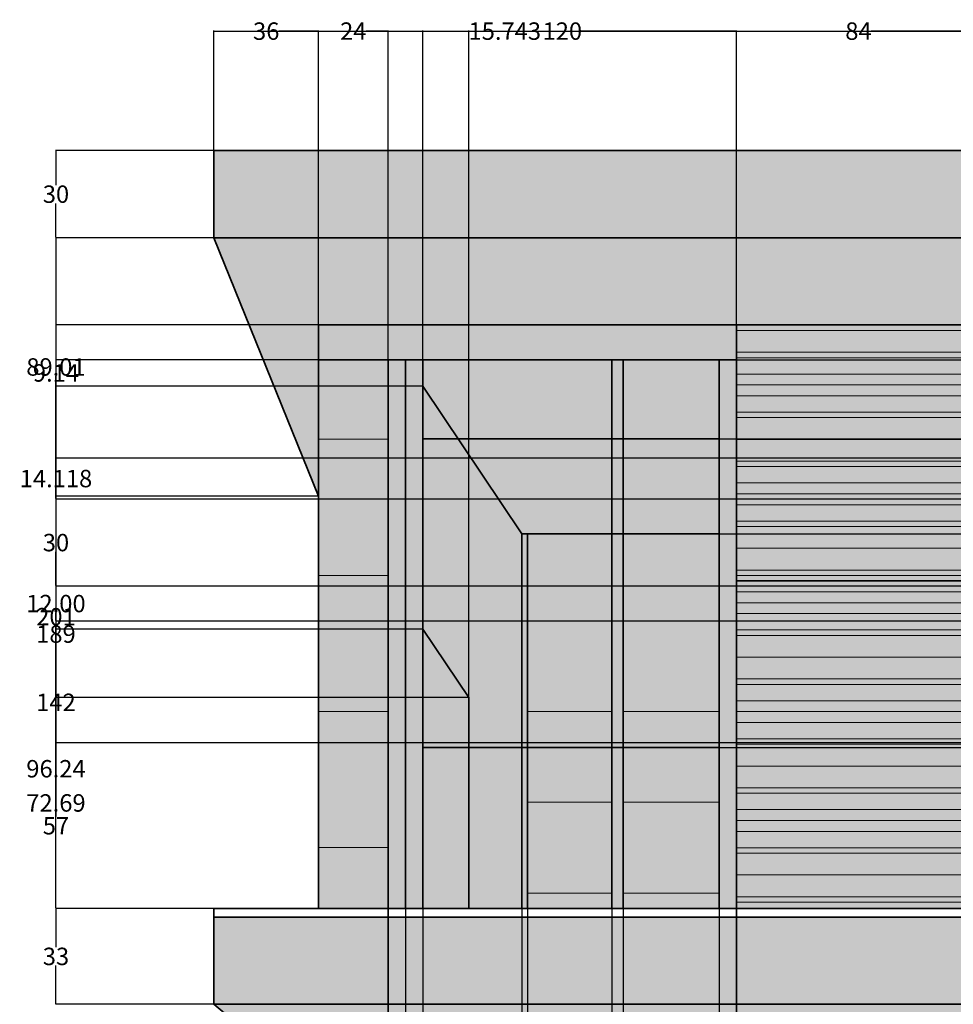
# Model space of a CAD drawing. Units: inches. Extents: x 148 to 1080, y 89 to 707.
# Tile 6 of 12: x 148 to 470, y 368 to 707. Entities that reach past the tile are written whole.
import ezdxf

# ---------------------------------------------------------------- set-up
doc = ezdxf.new("R2010")
doc.units = ezdxf.units.IN
doc.header["$MEASUREMENT"] = 0
for name, color, linetype, lineweight in [('A-ANNO-DIMS', 2, 'Continuous', 18), ('A-ELEV', 7, 'Continuous', 35), ('A-ELEV-PATT', 8, 'Continuous', 13)]:
    doc.layers.add(name, color=color, linetype=linetype, lineweight=lineweight)
doc.styles.get("Standard").update_dxf_attribs({"font": 'arial.ttf'})
doc.dimstyles.get("Standard").update_dxf_attribs({"dimtxt": 6, "dimasz": 0.18, "dimexe": 0.18, "dimexo": 0.0625, "dimgap": 0.09, "dimtad": 0, "dimtih": 1, "dimtoh": 1, "dimdec": 0, "dimzin": 0, "dimdsep": 46, "dimlunit": 3, "dimtxsty": 'Standard', "dimcen": 0.09, "dimadec": 0, "dimazin": 0, "dimtfac": 1, "dimtdec": 0, "dimtofl": 0, "dimtmove": 0, "dimatfit": 3, "dimfxl": 1, "dimtolj": 1, "dimtzin": 0, "dimarcsym": 0})

# ---------------------------------------------------------------- blocks, each defined once
blk = doc.blocks.new('*D1')
at = {"layer": 'A-ANNO-DIMS', "color": 0, "lineweight": -2, "transparency": 16777216}
for p, q in [((215.02, 662.01), (215.02, 703.28)), ((215.2, 703.1), (604.32, 703.1)), ((1006.77, 703.1), (617.65, 703.1)), ((1006.95, 338.01), (1006.95, 703.28))]:
    blk.add_line(p, q, dxfattribs=at)
at = {"layer": 'A-ANNO-DIMS', "color": 0, "transparency": 16777216}
for points in [[(215.2, 703.13), (215.2, 703.07), (215.02, 703.1)], [(1006.77, 703.13), (1006.77, 703.07), (1006.95, 703.1)]]:
    blk.add_solid(points, dxfattribs=at)
at = {"layer": 'Defpoints', "color": 0, "transparency": 16777216}
for p in [(1006.95, 703.1), (215.02, 661.95), (1006.95, 337.95)]:
    blk.add_point(p, dxfattribs=at)
at = {"layer": 'A-ANNO-DIMS', "color": 0, "transparency": 16777216, "insert": (610.98, 703.1), "char_height": 6, "attachment_point": 5}
blk.add_mtext('\\A1;792', dxfattribs=at)
blk = doc.blocks.new('*D8')
at = {"layer": 'A-ANNO-DIMS', "color": 0, "lineweight": -2, "transparency": 16777216}
for p, q in [((215.02, 632.01), (215.02, 703.28)), ((215.2, 703.1), (228.64, 703.1)), ((250.84, 703.1), (237.4, 703.1)), ((251.02, 543), (251.02, 703.28))]:
    blk.add_line(p, q, dxfattribs=at)
at = {"layer": 'A-ANNO-DIMS', "color": 0, "transparency": 16777216}
for points in [[(215.2, 703.13), (215.2, 703.07), (215.02, 703.1)], [(250.84, 703.13), (250.84, 703.07), (251.02, 703.1)]]:
    blk.add_solid(points, dxfattribs=at)
at = {"layer": 'Defpoints', "color": 0, "transparency": 16777216}
for p in [(251.02, 703.1), (215.02, 631.95), (251.02, 542.94)]:
    blk.add_point(p, dxfattribs=at)
at = {"layer": 'A-ANNO-DIMS', "color": 0, "transparency": 16777216, "insert": (233.02, 703.1), "char_height": 6, "attachment_point": 5}
blk.add_mtext('\\A1;36', dxfattribs=at)
blk = doc.blocks.new('*D9')
at = {"layer": 'A-ANNO-DIMS', "color": 0, "lineweight": -2, "transparency": 16777216}
for p, q in [((251.02, 602.01), (251.02, 703.28)), ((251.2, 703.1), (258.59, 703.1)), ((274.84, 703.1), (267.45, 703.1)), ((275.02, 590.01), (275.02, 703.28))]:
    blk.add_line(p, q, dxfattribs=at)
at = {"layer": 'A-ANNO-DIMS', "color": 0, "transparency": 16777216}
for points in [[(251.2, 703.13), (251.2, 703.07), (251.02, 703.1)], [(274.84, 703.13), (274.84, 703.07), (275.02, 703.1)]]:
    blk.add_solid(points, dxfattribs=at)
at = {"layer": 'Defpoints', "color": 0, "transparency": 16777216}
for p in [(275.02, 703.1), (251.02, 601.95), (275.02, 589.95)]:
    blk.add_point(p, dxfattribs=at)
at = {"layer": 'A-ANNO-DIMS', "color": 0, "transparency": 16777216, "insert": (263.02, 703.1), "char_height": 6, "attachment_point": 5}
blk.add_mtext('\\A1;24', dxfattribs=at)
blk = doc.blocks.new('*D10')
at = {"layer": 'A-ANNO-DIMS', "color": 0, "lineweight": -2, "transparency": 16777216}
for p, q in [((275.02, 590.01), (275.02, 703.28)), ((275.2, 703.1), (328.59, 703.1)), ((394.84, 703.1), (341.45, 703.1)), ((395.02, 590.01), (395.02, 703.28))]:
    blk.add_line(p, q, dxfattribs=at)
at = {"layer": 'A-ANNO-DIMS', "color": 0, "transparency": 16777216}
for points in [[(275.2, 703.13), (275.2, 703.07), (275.02, 703.1)], [(394.84, 703.13), (394.84, 703.07), (395.02, 703.1)]]:
    blk.add_solid(points, dxfattribs=at)
at = {"layer": 'Defpoints', "color": 0, "transparency": 16777216}
for p in [(395.02, 703.1), (275.02, 589.95), (395.02, 589.95)]:
    blk.add_point(p, dxfattribs=at)
at = {"layer": 'A-ANNO-DIMS', "color": 0, "transparency": 16777216, "insert": (335.02, 703.1), "char_height": 6, "attachment_point": 5}
blk.add_mtext('\\A1;120', dxfattribs=at)
blk = doc.blocks.new('*D11')
at = {"layer": 'A-ANNO-DIMS', "color": 0, "lineweight": -2, "transparency": 16777216}
for p, q in [((395.02, 602.01), (395.02, 703.28)), ((395.2, 703.1), (432.64, 703.1)), ((478.84, 703.1), (441.4, 703.1)), ((479.02, 602.01), (479.02, 703.28))]:
    blk.add_line(p, q, dxfattribs=at)
at = {"layer": 'A-ANNO-DIMS', "color": 0, "transparency": 16777216}
for points in [[(395.2, 703.13), (395.2, 703.07), (395.02, 703.1)], [(478.84, 703.13), (478.84, 703.07), (479.02, 703.1)]]:
    blk.add_solid(points, dxfattribs=at)
at = {"layer": 'Defpoints', "color": 0, "transparency": 16777216}
for p in [(479.02, 703.1), (395.02, 601.95), (479.02, 601.95)]:
    blk.add_point(p, dxfattribs=at)
at = {"layer": 'A-ANNO-DIMS', "color": 0, "transparency": 16777216, "insert": (437.02, 703.1), "char_height": 6, "attachment_point": 5}
blk.add_mtext('\\A1;84', dxfattribs=at)
blk = doc.blocks.new('*D19')
at = {"layer": 'A-ANNO-DIMS', "color": 0, "lineweight": -2, "transparency": 16777216}
for p, q in [((214.96, 661.95), (160.42, 661.95)), ((160.6, 661.77), (160.6, 650.1)), ((160.6, 632.13), (160.6, 643.79)), ((214.96, 631.95), (160.42, 631.95))]:
    blk.add_line(p, q, dxfattribs=at)
at = {"layer": 'A-ANNO-DIMS', "color": 0, "transparency": 16777216}
for points in [[(160.57, 661.77), (160.63, 661.77), (160.6, 661.95)], [(160.57, 632.13), (160.63, 632.13), (160.6, 631.95)]]:
    blk.add_solid(points, dxfattribs=at)
at = {"layer": 'Defpoints', "color": 0, "transparency": 16777216}
for p in [(215.02, 661.95), (160.6, 631.95), (215.02, 631.95)]:
    blk.add_point(p, dxfattribs=at)
at = {"layer": 'A-ANNO-DIMS', "color": 0, "transparency": 16777216, "insert": (160.6, 646.95), "char_height": 6, "attachment_point": 5}
blk.add_mtext('\\A1;30', dxfattribs=at)
blk = doc.blocks.new('*D20')
at = {"layer": 'A-ANNO-DIMS', "color": 0, "lineweight": -2, "transparency": 16777216}
for p, q in [((214.96, 631.95), (160.42, 631.95)), ((160.6, 631.77), (160.6, 590.59)), ((160.6, 543.12), (160.6, 584.29)), ((250.96, 542.94), (160.42, 542.94))]:
    blk.add_line(p, q, dxfattribs=at)
at = {"layer": 'A-ANNO-DIMS', "color": 0, "transparency": 16777216}
for points in [[(160.57, 631.77), (160.63, 631.77), (160.6, 631.95)], [(160.57, 543.12), (160.63, 543.12), (160.6, 542.94)]]:
    blk.add_solid(points, dxfattribs=at)
at = {"layer": 'Defpoints', "color": 0, "transparency": 16777216}
for p in [(215.02, 631.95), (160.6, 542.94), (251.02, 542.94)]:
    blk.add_point(p, dxfattribs=at)
at = {"layer": 'A-ANNO-DIMS', "color": 0, "transparency": 16777216, "insert": (160.6, 587.44), "char_height": 6, "attachment_point": 5}
blk.add_mtext('\\A1;89.01', dxfattribs=at)
blk = doc.blocks.new('*D21')
at = {"layer": 'A-ANNO-DIMS', "color": 0, "lineweight": -2, "transparency": 16777216}
for p, q in [((250.96, 542.94), (160.42, 542.94)), ((160.6, 542.76), (160.6, 475.04)), ((160.6, 401.13), (160.6, 468.84)), ((214.96, 400.95), (160.42, 400.95))]:
    blk.add_line(p, q, dxfattribs=at)
at = {"layer": 'A-ANNO-DIMS', "color": 0, "transparency": 16777216}
for points in [[(160.57, 542.76), (160.63, 542.76), (160.6, 542.94)], [(160.57, 401.13), (160.63, 401.13), (160.6, 400.95)]]:
    blk.add_solid(points, dxfattribs=at)
at = {"layer": 'Defpoints', "color": 0, "transparency": 16777216}
for p in [(251.02, 542.94), (160.6, 400.95), (215.02, 400.95)]:
    blk.add_point(p, dxfattribs=at)
at = {"layer": 'A-ANNO-DIMS', "color": 0, "transparency": 16777216, "insert": (160.6, 471.94), "char_height": 6, "attachment_point": 5}
blk.add_mtext('\\A1;142', dxfattribs=at)
blk = doc.blocks.new('*D22')
at = {"layer": 'A-ANNO-DIMS', "color": 0, "lineweight": -2, "transparency": 16777216}
for p, q in [((214.96, 400.95), (160.42, 400.95)), ((160.6, 400.77), (160.6, 387.6)), ((160.6, 368.13), (160.6, 381.29)), ((214.96, 367.95), (160.42, 367.95))]:
    blk.add_line(p, q, dxfattribs=at)
at = {"layer": 'A-ANNO-DIMS', "color": 0, "transparency": 16777216}
for points in [[(160.57, 400.77), (160.63, 400.77), (160.6, 400.95)], [(160.57, 368.13), (160.63, 368.13), (160.6, 367.95)]]:
    blk.add_solid(points, dxfattribs=at)
at = {"layer": 'Defpoints', "color": 0, "transparency": 16777216}
for p in [(215.02, 400.95), (160.6, 367.95), (215.02, 367.95)]:
    blk.add_point(p, dxfattribs=at)
at = {"layer": 'A-ANNO-DIMS', "color": 0, "transparency": 16777216, "insert": (160.6, 384.45), "char_height": 6, "attachment_point": 5}
blk.add_mtext('\\A1;33', dxfattribs=at)
blk = doc.blocks.new('*D25')
at = {"layer": 'A-ANNO-DIMS', "color": 0, "lineweight": -2, "transparency": 16777216}
for p, q in [((250.96, 601.95), (160.42, 601.95)), ((160.6, 601.77), (160.6, 504.6)), ((160.6, 401.13), (160.6, 498.29)), ((250.96, 400.95), (160.42, 400.95))]:
    blk.add_line(p, q, dxfattribs=at)
at = {"layer": 'A-ANNO-DIMS', "color": 0, "transparency": 16777216}
for points in [[(160.57, 601.77), (160.63, 601.77), (160.6, 601.95)], [(160.57, 401.13), (160.63, 401.13), (160.6, 400.95)]]:
    blk.add_solid(points, dxfattribs=at)
at = {"layer": 'Defpoints', "color": 0, "transparency": 16777216}
for p in [(251.02, 601.95), (160.6, 400.95), (251.02, 400.95)]:
    blk.add_point(p, dxfattribs=at)
at = {"layer": 'A-ANNO-DIMS', "color": 0, "transparency": 16777216, "insert": (160.6, 501.45), "char_height": 6, "attachment_point": 5}
blk.add_mtext('\\A1;201', dxfattribs=at)
blk = doc.blocks.new('*D26')
at = {"layer": 'A-ANNO-DIMS', "color": 0, "lineweight": -2, "transparency": 16777216}
for p, q in [((274.96, 589.95), (160.42, 589.95)), ((160.6, 589.77), (160.6, 498.6)), ((160.6, 401.13), (160.6, 492.29)), ((274.96, 400.95), (160.42, 400.95))]:
    blk.add_line(p, q, dxfattribs=at)
at = {"layer": 'A-ANNO-DIMS', "color": 0, "transparency": 16777216}
for points in [[(160.57, 589.77), (160.63, 589.77), (160.6, 589.95)], [(160.57, 401.13), (160.63, 401.13), (160.6, 400.95)]]:
    blk.add_solid(points, dxfattribs=at)
at = {"layer": 'Defpoints', "color": 0, "transparency": 16777216}
for p in [(160.6, 589.95), (275.02, 589.95), (275.02, 400.95)]:
    blk.add_point(p, dxfattribs=at)
at = {"layer": 'A-ANNO-DIMS', "color": 0, "transparency": 16777216, "insert": (160.6, 495.45), "char_height": 6, "attachment_point": 5}
blk.add_mtext('\\A1;189', dxfattribs=at)
blk = doc.blocks.new('*D27')
at = {"layer": 'A-ANNO-DIMS', "color": 0, "lineweight": -2, "transparency": 16777216}
for p, q in [((275.02, 332.01), (275.02, 703.28)), ((275.2, 703.1), (328.59, 703.1)), ((394.84, 703.1), (341.45, 703.1)), ((395.02, 332.01), (395.02, 703.28))]:
    blk.add_line(p, q, dxfattribs=at)
at = {"layer": 'A-ANNO-DIMS', "color": 0, "transparency": 16777216}
for points in [[(275.2, 703.13), (275.2, 703.07), (275.02, 703.1)], [(394.84, 703.13), (394.84, 703.07), (395.02, 703.1)]]:
    blk.add_solid(points, dxfattribs=at)
at = {"layer": 'Defpoints', "color": 0, "transparency": 16777216}
for p in [(395.02, 703.1), (275.02, 331.95), (395.02, 331.95)]:
    blk.add_point(p, dxfattribs=at)
at = {"layer": 'A-ANNO-DIMS', "color": 0, "transparency": 16777216, "insert": (335.02, 703.1), "char_height": 6, "attachment_point": 5}
blk.add_mtext('\\A1;120', dxfattribs=at)
blk = doc.blocks.new('*D40')
at = {"layer": 'A-ANNO-DIMS', "color": 0, "lineweight": -2, "transparency": 16777216}
for p, q in [((526.96, 457.95), (160.42, 457.95)), ((160.6, 457.77), (160.6, 432.59)), ((160.6, 401.13), (160.6, 426.31)), ((526.96, 400.95), (160.42, 400.95))]:
    blk.add_line(p, q, dxfattribs=at)
at = {"layer": 'A-ANNO-DIMS', "color": 0, "transparency": 16777216}
for points in [[(160.57, 457.77), (160.63, 457.77), (160.6, 457.95)], [(160.57, 401.13), (160.63, 401.13), (160.6, 400.95)]]:
    blk.add_solid(points, dxfattribs=at)
at = {"layer": 'Defpoints', "color": 0, "transparency": 16777216}
for p in [(527.02, 457.95), (160.6, 400.95), (527.02, 400.95)]:
    blk.add_point(p, dxfattribs=at)
at = {"layer": 'A-ANNO-DIMS', "color": 0, "transparency": 16777216, "insert": (160.6, 429.45), "char_height": 6, "attachment_point": 5}
blk.add_mtext('\\A1;57', dxfattribs=at)
blk = doc.blocks.new('*D41')
at = {"layer": 'A-ANNO-DIMS', "color": 0, "lineweight": -2, "transparency": 16777216}
for p, q in [((610.96, 541.95), (160.42, 541.95)), ((160.6, 541.77), (160.6, 530.1)), ((160.6, 512.13), (160.6, 523.79)), ((610.96, 511.95), (160.42, 511.95))]:
    blk.add_line(p, q, dxfattribs=at)
at = {"layer": 'A-ANNO-DIMS', "color": 0, "transparency": 16777216}
for points in [[(160.57, 541.77), (160.63, 541.77), (160.6, 541.95)], [(160.57, 512.13), (160.63, 512.13), (160.6, 511.95)]]:
    blk.add_solid(points, dxfattribs=at)
at = {"layer": 'Defpoints', "color": 0, "transparency": 16777216}
for p in [(611.02, 541.95), (160.6, 511.95), (611.02, 511.95)]:
    blk.add_point(p, dxfattribs=at)
at = {"layer": 'A-ANNO-DIMS', "color": 0, "transparency": 16777216, "insert": (160.6, 526.95), "char_height": 6, "attachment_point": 5}
blk.add_mtext('\\A1;30', dxfattribs=at)
blk = doc.blocks.new('*D46')
at = {"layer": 'A-ANNO-DIMS', "color": 0, "lineweight": -2, "transparency": 16777216}
for p, q in [((583.7, 556.07), (160.42, 556.07)), ((160.6, 555.89), (160.6, 552.16)), ((160.6, 542.13), (160.6, 545.85)), ((598.54, 541.95), (160.42, 541.95))]:
    blk.add_line(p, q, dxfattribs=at)
at = {"layer": 'A-ANNO-DIMS', "color": 0, "transparency": 16777216}
for points in [[(160.57, 555.89), (160.63, 555.89), (160.6, 556.07)], [(160.57, 542.13), (160.63, 542.13), (160.6, 541.95)]]:
    blk.add_solid(points, dxfattribs=at)
at = {"layer": 'Defpoints', "color": 0, "transparency": 16777216}
for p in [(583.76, 556.07), (160.6, 541.95), (598.6, 541.95)]:
    blk.add_point(p, dxfattribs=at)
at = {"layer": 'A-ANNO-DIMS', "color": 0, "transparency": 16777216, "insert": (160.6, 549.01), "char_height": 6, "attachment_point": 5}
blk.add_mtext('\\A1;14.118', dxfattribs=at)
blk = doc.blocks.new('*D52')
at = {"layer": 'A-ANNO-DIMS', "color": 0, "lineweight": -2, "transparency": 16777216}
for p, q in [((610.96, 511.95), (160.42, 511.95)), ((160.6, 511.77), (160.6, 509.1)), ((160.6, 500.13), (160.6, 502.79)), ((610.96, 499.95), (160.42, 499.95))]:
    blk.add_line(p, q, dxfattribs=at)
at = {"layer": 'A-ANNO-DIMS', "color": 0, "transparency": 16777216}
for points in [[(160.57, 511.77), (160.63, 511.77), (160.6, 511.95)], [(160.57, 500.13), (160.63, 500.13), (160.6, 499.95)]]:
    blk.add_solid(points, dxfattribs=at)
at = {"layer": 'Defpoints', "color": 0, "transparency": 16777216}
for p in [(160.6, 511.95), (611.02, 511.95), (611.02, 499.95)]:
    blk.add_point(p, dxfattribs=at)
at = {"layer": 'A-ANNO-DIMS', "color": 0, "transparency": 16777216, "insert": (160.6, 505.95), "char_height": 6, "attachment_point": 5}
blk.add_mtext('\\A1;12.00', dxfattribs=at)
blk = doc.blocks.new('*D82')
at = {"layer": 'A-ANNO-DIMS', "color": 0, "lineweight": -2, "transparency": 16777216}
for p, q in [((275.02, 400.88), (275.02, 92.62)), ((281.02, 400.88), (281.02, 92.62)), ((275.2, 92.8), (280.84, 92.8)), ((281.02, 92.8), (281.2, 92.8))]:
    blk.add_line(p, q, dxfattribs=at)
at = {"layer": 'A-ANNO-DIMS', "color": 0, "transparency": 16777216}
for points in [[(275.2, 92.83), (275.2, 92.77), (275.02, 92.8)], [(280.84, 92.83), (280.84, 92.77), (281.02, 92.8)]]:
    blk.add_solid(points, dxfattribs=at)
at = {"layer": 'Defpoints', "color": 0, "transparency": 16777216}
for p in [(275.02, 400.95), (281.02, 400.95), (281.02, 92.8)]:
    blk.add_point(p, dxfattribs=at)
at = {"layer": 'A-ANNO-DIMS', "color": 0, "transparency": 16777216, "insert": (289.09, 92.8), "char_height": 6, "attachment_point": 5}
blk.add_mtext('\\A1;6.00', dxfattribs=at)
blk = doc.blocks.new('*D83')
at = {"layer": 'A-ANNO-DIMS', "color": 0, "lineweight": -2, "transparency": 16777216}
for p, q in [((281.02, 400.88), (281.02, 92.62)), ((287.02, 400.88), (287.02, 92.62)), ((281.2, 92.8), (286.84, 92.8)), ((287.02, 92.8), (287.2, 92.8))]:
    blk.add_line(p, q, dxfattribs=at)
at = {"layer": 'A-ANNO-DIMS', "color": 0, "transparency": 16777216}
for points in [[(281.2, 92.83), (281.2, 92.77), (281.02, 92.8)], [(286.84, 92.83), (286.84, 92.77), (287.02, 92.8)]]:
    blk.add_solid(points, dxfattribs=at)
at = {"layer": 'Defpoints', "color": 0, "transparency": 16777216}
for p in [(281.02, 400.95), (287.02, 400.95), (287.02, 92.8)]:
    blk.add_point(p, dxfattribs=at)
at = {"layer": 'A-ANNO-DIMS', "color": 0, "transparency": 16777216, "insert": (295.09, 92.8), "char_height": 6, "attachment_point": 5}
blk.add_mtext('\\A1;6.00', dxfattribs=at)
blk = doc.blocks.new('*D84')
at = {"layer": 'A-ANNO-DIMS', "color": 0, "lineweight": -2, "transparency": 16777216}
for p, q in [((321.02, 529.88), (321.02, 92.62)), ((287.02, 400.88), (287.02, 92.62)), ((287.2, 92.8), (293.82, 92.8)), ((320.84, 92.8), (314.22, 92.8))]:
    blk.add_line(p, q, dxfattribs=at)
at = {"layer": 'A-ANNO-DIMS', "color": 0, "transparency": 16777216}
for points in [[(287.2, 92.83), (287.2, 92.77), (287.02, 92.8)], [(320.84, 92.83), (320.84, 92.77), (321.02, 92.8)]]:
    blk.add_solid(points, dxfattribs=at)
at = {"layer": 'Defpoints', "color": 0, "transparency": 16777216}
for p in [(321.02, 529.95), (287.02, 400.95), (321.02, 92.8)]:
    blk.add_point(p, dxfattribs=at)
at = {"layer": 'A-ANNO-DIMS', "color": 0, "transparency": 16777216, "insert": (304.02, 92.8), "char_height": 6, "attachment_point": 5}
blk.add_mtext('\\A1;34.00', dxfattribs=at)
blk = doc.blocks.new('*D85')
at = {"layer": 'A-ANNO-DIMS', "color": 0, "lineweight": -2, "transparency": 16777216}
for p, q in [((321.02, 529.88), (321.02, 92.62)), ((323.02, 400.88), (323.02, 92.62)), ((321.2, 92.8), (322.84, 92.8)), ((323.02, 92.8), (323.2, 92.8))]:
    blk.add_line(p, q, dxfattribs=at)
at = {"layer": 'A-ANNO-DIMS', "color": 0, "transparency": 16777216}
for points in [[(321.2, 92.83), (321.2, 92.77), (321.02, 92.8)], [(322.84, 92.83), (322.84, 92.77), (323.02, 92.8)]]:
    blk.add_solid(points, dxfattribs=at)
at = {"layer": 'Defpoints', "color": 0, "transparency": 16777216}
for p in [(321.02, 529.95), (323.02, 400.95), (323.02, 92.8)]:
    blk.add_point(p, dxfattribs=at)
at = {"layer": 'A-ANNO-DIMS', "color": 0, "transparency": 16777216, "insert": (331.12, 92.8), "char_height": 6, "attachment_point": 5}
blk.add_mtext('\\A1;2.00', dxfattribs=at)
blk = doc.blocks.new('*D86')
at = {"layer": 'A-ANNO-DIMS', "color": 0, "lineweight": -2, "transparency": 16777216}
for p, q in [((323.02, 400.88), (323.02, 92.62)), ((352.02, 400.88), (352.02, 92.62)), ((323.2, 92.8), (327.27, 92.8)), ((351.84, 92.8), (347.77, 92.8))]:
    blk.add_line(p, q, dxfattribs=at)
at = {"layer": 'A-ANNO-DIMS', "color": 0, "transparency": 16777216}
for points in [[(323.2, 92.83), (323.2, 92.77), (323.02, 92.8)], [(351.84, 92.83), (351.84, 92.77), (352.02, 92.8)]]:
    blk.add_solid(points, dxfattribs=at)
at = {"layer": 'Defpoints', "color": 0, "transparency": 16777216}
for p in [(323.02, 400.95), (352.02, 400.95), (352.02, 92.8)]:
    blk.add_point(p, dxfattribs=at)
at = {"layer": 'A-ANNO-DIMS', "color": 0, "transparency": 16777216, "insert": (337.52, 92.8), "char_height": 6, "attachment_point": 5}
blk.add_mtext('\\A1;29.00', dxfattribs=at)
blk = doc.blocks.new('*D87')
at = {"layer": 'A-ANNO-DIMS', "color": 0, "lineweight": -2, "transparency": 16777216}
for p, q in [((352.02, 400.88), (352.02, 92.62)), ((356.02, 400.88), (356.02, 92.62)), ((352.2, 92.8), (355.84, 92.8)), ((356.02, 92.8), (356.2, 92.8))]:
    blk.add_line(p, q, dxfattribs=at)
at = {"layer": 'A-ANNO-DIMS', "color": 0, "transparency": 16777216}
for points in [[(352.2, 92.83), (352.2, 92.77), (352.02, 92.8)], [(355.84, 92.83), (355.84, 92.77), (356.02, 92.8)]]:
    blk.add_solid(points, dxfattribs=at)
at = {"layer": 'Defpoints', "color": 0, "transparency": 16777216}
for p in [(352.02, 400.95), (356.02, 400.95), (356.02, 92.8)]:
    blk.add_point(p, dxfattribs=at)
at = {"layer": 'A-ANNO-DIMS', "color": 0, "transparency": 16777216, "insert": (364.19, 92.8), "char_height": 6, "attachment_point": 5}
blk.add_mtext('\\A1;4.00', dxfattribs=at)
blk = doc.blocks.new('*D88')
at = {"layer": 'A-ANNO-DIMS', "color": 0, "lineweight": -2, "transparency": 16777216}
for p, q in [((356.02, 400.88), (356.02, 92.62)), ((389.02, 400.88), (389.02, 92.62)), ((356.2, 92.8), (362.32, 92.8)), ((388.84, 92.8), (382.72, 92.8))]:
    blk.add_line(p, q, dxfattribs=at)
at = {"layer": 'A-ANNO-DIMS', "color": 0, "transparency": 16777216}
for points in [[(356.2, 92.83), (356.2, 92.77), (356.02, 92.8)], [(388.84, 92.83), (388.84, 92.77), (389.02, 92.8)]]:
    blk.add_solid(points, dxfattribs=at)
at = {"layer": 'Defpoints', "color": 0, "transparency": 16777216}
for p in [(356.02, 400.95), (389.02, 400.95), (389.02, 92.8)]:
    blk.add_point(p, dxfattribs=at)
at = {"layer": 'A-ANNO-DIMS', "color": 0, "transparency": 16777216, "insert": (372.52, 92.8), "char_height": 6, "attachment_point": 5}
blk.add_mtext('\\A1;33.00', dxfattribs=at)
blk = doc.blocks.new('*D89')
at = {"layer": 'A-ANNO-DIMS', "color": 0, "lineweight": -2, "transparency": 16777216}
for p, q in [((389.02, 400.88), (389.02, 92.62)), ((395.02, 400.88), (395.02, 92.62)), ((389.2, 92.8), (394.84, 92.8)), ((395.02, 92.8), (395.2, 92.8))]:
    blk.add_line(p, q, dxfattribs=at)
at = {"layer": 'A-ANNO-DIMS', "color": 0, "transparency": 16777216}
for points in [[(389.2, 92.83), (389.2, 92.77), (389.02, 92.8)], [(394.84, 92.83), (394.84, 92.77), (395.02, 92.8)]]:
    blk.add_solid(points, dxfattribs=at)
at = {"layer": 'Defpoints', "color": 0, "transparency": 16777216}
for p in [(389.02, 400.95), (395.02, 400.95), (395.02, 92.8)]:
    blk.add_point(p, dxfattribs=at)
at = {"layer": 'A-ANNO-DIMS', "color": 0, "transparency": 16777216, "insert": (403.09, 92.8), "char_height": 6, "attachment_point": 5}
blk.add_mtext('\\A1;6.00', dxfattribs=at)
blk = doc.blocks.new('*D92')
at = {"layer": 'A-ANNO-DIMS', "color": 0, "lineweight": -2, "transparency": 16777216}
for p, q in [((389.08, 456.43), (1064.5, 456.43)), ((1064.32, 456.25), (1064.32, 431.84)), ((1064.32, 401.13), (1064.32, 425.53)), ((389.08, 400.95), (1064.5, 400.95))]:
    blk.add_line(p, q, dxfattribs=at)
at = {"layer": 'A-ANNO-DIMS', "color": 0, "transparency": 16777216}
for points in [[(1064.29, 456.25), (1064.35, 456.25), (1064.32, 456.43)], [(1064.29, 401.13), (1064.35, 401.13), (1064.32, 400.95)]]:
    blk.add_solid(points, dxfattribs=at)
at = {"layer": 'Defpoints', "color": 0, "transparency": 16777216}
for p in [(389.02, 456.43), (1064.32, 456.43), (389.02, 400.95)]:
    blk.add_point(p, dxfattribs=at)
at = {"layer": 'A-ANNO-DIMS', "color": 0, "transparency": 16777216, "insert": (1064.32, 428.69), "char_height": 6, "attachment_point": 5}
blk.add_mtext('\\A1;55.48', dxfattribs=at)
blk = doc.blocks.new('*D93')
at = {"layer": 'A-ANNO-DIMS', "color": 0, "lineweight": -2, "transparency": 16777216}
for p, q in [((389.08, 529.95), (1064.5, 529.95)), ((1064.32, 529.77), (1064.32, 496.34)), ((1064.32, 456.61), (1064.32, 490.03)), ((389.08, 456.43), (1064.5, 456.43))]:
    blk.add_line(p, q, dxfattribs=at)
at = {"layer": 'A-ANNO-DIMS', "color": 0, "transparency": 16777216}
for points in [[(1064.29, 529.77), (1064.35, 529.77), (1064.32, 529.95)], [(1064.29, 456.61), (1064.35, 456.61), (1064.32, 456.43)]]:
    blk.add_solid(points, dxfattribs=at)
at = {"layer": 'Defpoints', "color": 0, "transparency": 16777216}
for p in [(389.02, 529.95), (1064.32, 529.95), (389.02, 456.43)]:
    blk.add_point(p, dxfattribs=at)
at = {"layer": 'A-ANNO-DIMS', "color": 0, "transparency": 16777216, "insert": (1064.32, 493.19), "char_height": 6, "attachment_point": 5}
blk.add_mtext('\\A1;73.52', dxfattribs=at)
blk = doc.blocks.new('*D94')
at = {"layer": 'A-ANNO-DIMS', "color": 0, "lineweight": -2, "transparency": 16777216}
for p, q in [((389.08, 562.74), (1064.5, 562.74)), ((1064.32, 562.56), (1064.32, 549.5)), ((1064.32, 530.13), (1064.32, 543.19)), ((389.08, 529.95), (1064.5, 529.95))]:
    blk.add_line(p, q, dxfattribs=at)
at = {"layer": 'A-ANNO-DIMS', "color": 0, "transparency": 16777216}
for points in [[(1064.29, 562.56), (1064.35, 562.56), (1064.32, 562.74)], [(1064.29, 530.13), (1064.35, 530.13), (1064.32, 529.95)]]:
    blk.add_solid(points, dxfattribs=at)
at = {"layer": 'Defpoints', "color": 0, "transparency": 16777216}
for p in [(389.02, 562.74), (1064.32, 562.74), (389.02, 529.95)]:
    blk.add_point(p, dxfattribs=at)
at = {"layer": 'A-ANNO-DIMS', "color": 0, "transparency": 16777216, "insert": (1064.32, 546.34), "char_height": 6, "attachment_point": 5}
blk.add_mtext('\\A1;32.79', dxfattribs=at)
blk = doc.blocks.new('*D95')
at = {"layer": 'A-ANNO-DIMS', "color": 0, "lineweight": -2, "transparency": 16777216}
for p, q in [((389.08, 589.95), (1064.5, 589.95)), ((1064.32, 589.77), (1064.32, 579.44)), ((1064.32, 562.92), (1064.32, 573.24)), ((389.08, 562.74), (1064.5, 562.74))]:
    blk.add_line(p, q, dxfattribs=at)
at = {"layer": 'A-ANNO-DIMS', "color": 0, "transparency": 16777216}
for points in [[(1064.29, 589.77), (1064.35, 589.77), (1064.32, 589.95)], [(1064.29, 562.92), (1064.35, 562.92), (1064.32, 562.74)]]:
    blk.add_solid(points, dxfattribs=at)
at = {"layer": 'Defpoints', "color": 0, "transparency": 16777216}
for p in [(389.02, 589.95), (1064.32, 589.95), (389.02, 562.74)]:
    blk.add_point(p, dxfattribs=at)
at = {"layer": 'A-ANNO-DIMS', "color": 0, "transparency": 16777216, "insert": (1064.32, 576.34), "char_height": 6, "attachment_point": 5}
blk.add_mtext('\\A1;27.21', dxfattribs=at)
blk = doc.blocks.new('*D96')
at = {"layer": 'A-ANNO-DIMS', "color": 0, "lineweight": -2, "transparency": 16777216}
for p, q in [((286.96, 589.95), (160.42, 589.95)), ((160.6, 589.77), (160.6, 588.53)), ((286.96, 580.81), (160.42, 580.81)), ((160.6, 580.99), (160.6, 582.22))]:
    blk.add_line(p, q, dxfattribs=at)
at = {"layer": 'A-ANNO-DIMS', "color": 0, "transparency": 16777216}
for points in [[(160.57, 589.77), (160.63, 589.77), (160.6, 589.95)], [(160.57, 580.99), (160.63, 580.99), (160.6, 580.81)]]:
    blk.add_solid(points, dxfattribs=at)
at = {"layer": 'Defpoints', "color": 0, "transparency": 16777216}
for p in [(160.6, 589.95), (287.02, 589.95), (287.02, 580.81)]:
    blk.add_point(p, dxfattribs=at)
at = {"layer": 'A-ANNO-DIMS', "color": 0, "transparency": 16777216, "insert": (160.6, 585.38), "char_height": 6, "attachment_point": 5}
blk.add_mtext('\\A1;9.14', dxfattribs=at)
blk = doc.blocks.new('*D97')
at = {"layer": 'A-ANNO-DIMS', "color": 0, "lineweight": -2, "transparency": 16777216}
for p, q in [((286.96, 497.19), (160.42, 497.19)), ((160.6, 497.01), (160.6, 452.22)), ((160.6, 401.13), (160.6, 445.92)), ((286.96, 400.95), (160.42, 400.95))]:
    blk.add_line(p, q, dxfattribs=at)
at = {"layer": 'A-ANNO-DIMS', "color": 0, "transparency": 16777216}
for points in [[(160.57, 497.01), (160.63, 497.01), (160.6, 497.19)], [(160.57, 401.13), (160.63, 401.13), (160.6, 400.95)]]:
    blk.add_solid(points, dxfattribs=at)
at = {"layer": 'Defpoints', "color": 0, "transparency": 16777216}
for p in [(287.02, 497.19), (160.6, 400.95), (287.02, 400.95)]:
    blk.add_point(p, dxfattribs=at)
at = {"layer": 'A-ANNO-DIMS', "color": 0, "transparency": 16777216, "insert": (160.6, 449.07), "char_height": 6, "attachment_point": 5}
blk.add_mtext('\\A1;96.24', dxfattribs=at)
blk = doc.blocks.new('*D98')
at = {"layer": 'A-ANNO-DIMS', "color": 0, "lineweight": -2, "transparency": 16777216}
for p, q in [((302.7, 473.64), (160.42, 473.64)), ((160.6, 473.46), (160.6, 440.45)), ((160.6, 401.13), (160.6, 434.14)), ((302.7, 400.95), (160.42, 400.95))]:
    blk.add_line(p, q, dxfattribs=at)
at = {"layer": 'A-ANNO-DIMS', "color": 0, "transparency": 16777216}
for points in [[(160.57, 473.46), (160.63, 473.46), (160.6, 473.64)], [(160.57, 401.13), (160.63, 401.13), (160.6, 400.95)]]:
    blk.add_solid(points, dxfattribs=at)
at = {"layer": 'Defpoints', "color": 0, "transparency": 16777216}
for p in [(302.76, 473.64), (160.6, 400.95), (302.76, 400.95)]:
    blk.add_point(p, dxfattribs=at)
at = {"layer": 'A-ANNO-DIMS', "color": 0, "transparency": 16777216, "insert": (160.6, 437.29), "char_height": 6, "attachment_point": 5}
blk.add_mtext('\\A1;72.69', dxfattribs=at)
blk = doc.blocks.new('*D99')
at = {"layer": 'A-ANNO-DIMS', "color": 0, "lineweight": -2, "transparency": 16777216}
for p, q in [((287.02, 497.25), (287.02, 703.28)), ((287.2, 703.1), (302.58, 703.1)), ((302.76, 473.7), (302.76, 703.28)), ((302.76, 703.1), (302.94, 703.1))]:
    blk.add_line(p, q, dxfattribs=at)
at = {"layer": 'A-ANNO-DIMS', "color": 0, "transparency": 16777216}
for points in [[(287.2, 703.13), (287.2, 703.07), (287.02, 703.1)], [(302.58, 703.13), (302.58, 703.07), (302.76, 703.1)]]:
    blk.add_solid(points, dxfattribs=at)
at = {"layer": 'Defpoints', "color": 0, "transparency": 16777216}
for p in [(302.76, 703.1), (287.02, 497.19), (302.76, 473.64)]:
    blk.add_point(p, dxfattribs=at)
at = {"layer": 'A-ANNO-DIMS', "color": 0, "transparency": 16777216, "insert": (315.2, 703.1), "char_height": 6, "attachment_point": 5}
blk.add_mtext('\\A1;15.743', dxfattribs=at)

msp = doc.modelspace()

# ---------------------------------------------------------------- hatches: boundary and pattern name
at = {"layer": 'A-ELEV-PATT'}
h = msp.add_hatch(color=256, dxfattribs=at)
h.dxf.hatch_style = 1
h.paths.add_polyline_path([(635.0199, 661.9474), (611.0199, 661.9474), (215.0199, 661.9474), (215.0199, 631.9474), (611.0199, 631.9474), (635.0199, 631.9474)])
h.paths.add_polyline_path([(773.0199, 397.9474), (215.0199, 397.9474), (215.0199, 367.9474), (773.0199, 367.9474)])
h = msp.add_hatch(color=256, dxfattribs=at)
h.dxf.hatch_style = 1
h.paths.add_polyline_path([(622.6005, 631.9474), (611.0199, 631.9474), (215.0199, 631.9474), (251.0199, 542.9352), (251.0199, 601.9474), (527.0199, 601.9474), (527.0199, 541.9474), (598.6005, 541.9474)])
h.paths.add_polyline_path([(558.5775, 608.9493, -1), (552.5775, 608.9493, -1)], flags=16)
h.paths.add_polyline_path([(586.7589, 556.0652, -1), (580.7589, 556.0652, -1)], flags=16)
h.paths.add_polyline_path([(635.0199, 631.9474), (622.6005, 631.9474), (598.6005, 541.9474), (611.0199, 541.9474)])
h.paths.add_polyline_path([(773.0199, 367.9474), (215.0199, 367.9474), (251.0199, 337.9474), (251.0199, 349.9474), (527.0199, 349.9474), (527.0199, 337.9474), (734.0628, 337.9474)])
h.paths.add_polyline_path([(631.1736, 353.1958, -1), (625.1736, 353.1958, -1)], flags=16)
h.paths.add_polyline_path([(729.9419, 354.8591, -1), (723.9419, 354.8591, -1)], flags=16)
h = msp.add_hatch(color=256, dxfattribs=at)
h.dxf.hatch_style = 1
h.paths.add_polyline_path([(395.0199, 349.9474), (275.0199, 349.9474), (275.0199, 331.9474), (395.0199, 331.9474)])
h.paths.add_polyline_path([(284.0199, 331.9474), (275.0199, 331.9474), (275.0199, 163.9474), (284.0199, 163.9474)])
h.paths.add_polyline_path([(395.0199, 601.9474), (251.0199, 601.9474), (251.0199, 589.9474), (395.0199, 589.9474)])
h = msp.add_hatch(color=256, dxfattribs=at)
h.dxf.hatch_style = 1
h.paths.add_polyline_path([(479.0199, 601.9474), (395.0199, 601.9474), (395.0199, 513.7706), (479.0199, 513.7706)])
h.paths.add_polyline_path([(527.0199, 489.89), (479.0199, 489.89), (479.0199, 400.9474), (527.0199, 400.9474)])
h = msp.add_hatch(dxfattribs=at)
h.set_pattern_fill('ANSI31', color=256, scale=60, angle=135)
h.paths.add_polyline_path([(479.0199, 601.9474), (395.0199, 601.9474), (395.0199, 513.7706), (479.0199, 513.7706)])
h.paths.add_polyline_path([(479.0199, 513.7706), (395.0199, 513.7706), (395.0199, 400.9474), (479.0199, 400.9474)])
h.paths.add_polyline_path([(683.0199, 337.9474), (527.0199, 337.9474), (527.0199, 283.9474), (683.0199, 283.9474)])
h = msp.add_hatch(dxfattribs=at)
h.set_pattern_fill('ANSI31', color=256, scale=75, angle=135)
h.paths.add_polyline_path([(479.0199, 601.9474), (395.0199, 601.9474), (395.0199, 513.7706), (479.0199, 513.7706)])
h.paths.add_polyline_path([(479.0199, 513.7706), (395.0199, 513.7706), (395.0199, 400.9474), (479.0199, 400.9474)])
h = msp.add_hatch(color=256, dxfattribs=at)
h.dxf.hatch_style = 1
h.paths.add_polyline_path([(275.0199, 589.9474), (251.0199, 589.9474), (251.0199, 400.9474), (275.0199, 400.9474)])
h = msp.add_hatch(dxfattribs=at)
h.set_pattern_fill('ANSI37', color=256, scale=375, angle=135)
h.paths.add_polyline_path([(275.0199, 589.9474), (251.0199, 589.9474), (251.0199, 400.9474), (275.0199, 400.9474)])
h = msp.add_hatch(color=256, dxfattribs=at)
h.dxf.hatch_style = 1
h.paths.add_polyline_path([(281.0199, 589.9474), (275.0199, 589.9474), (275.0199, 400.9474), (281.0199, 400.9474)])
h.paths.add_polyline_path([(287.0199, 589.9474), (281.0199, 589.9474), (281.0199, 400.9474), (287.0199, 400.9474)])
h.paths.add_polyline_path([(356.0199, 589.9474), (352.0199, 589.9474), (352.0199, 529.9474), (356.0199, 529.9474)])
h.paths.add_polyline_path([(356.0199, 529.9474), (352.0199, 529.9474), (352.0199, 400.9474), (356.0199, 400.9474)])
h.paths.add_polyline_path([(395.0199, 589.9474), (389.0199, 589.9474), (389.0199, 400.9474), (395.0199, 400.9474)])
h = msp.add_hatch(color=256, dxfattribs=at)
h.dxf.hatch_style = 1
h.paths.add_polyline_path([(352.0199, 456.4274), (323.0199, 456.4274), (323.0199, 400.9474), (352.0199, 400.9474)])
h.paths.add_polyline_path([(321.0199, 456.4274), (302.7628, 456.4274), (302.7628, 400.9474), (321.0199, 400.9474)])
h.paths.add_polyline_path([(321.0199, 529.9474), (299.1005, 562.736), (287.0199, 562.736), (287.0199, 497.1899), (302.7628, 473.6405), (302.7628, 456.4274), (321.0199, 456.4274)])
h.paths.add_polyline_path([(287.0199, 580.807), (287.0199, 562.736), (299.1005, 562.736)], flags=17)
h.paths.add_polyline_path([(352.0199, 589.9474), (287.0199, 589.9474), (287.0199, 580.807), (299.1005, 562.736), (352.0199, 562.736)])
h.paths.add_polyline_path([(352.0199, 562.736), (299.1005, 562.736), (321.0199, 529.9474), (352.0199, 529.9474)])
h.paths.add_polyline_path([(352.0199, 529.9474), (323.0199, 529.9474), (323.0199, 456.4274), (352.0199, 456.4274)])
h.paths.add_polyline_path([(389.0199, 529.9474), (356.0199, 529.9474), (356.0199, 456.4274), (389.0199, 456.4274)])
h.paths.add_polyline_path([(389.0199, 562.736), (356.0199, 562.736), (356.0199, 529.9474), (389.0199, 529.9474)])
h.paths.add_polyline_path([(389.0199, 589.9474), (356.0199, 589.9474), (356.0199, 562.736), (389.0199, 562.736)])
h.paths.add_polyline_path([(389.0199, 456.4274), (356.0199, 456.4274), (356.0199, 400.9474), (389.0199, 400.9474)])
h = msp.add_hatch(color=256, dxfattribs=at)
h.dxf.hatch_style = 1
h.paths.add_polyline_path([(707.0199, 511.9474), (707.0199, 541.9474), (611.0199, 541.9474), (611.0199, 511.9474)])
h.paths.add_polyline_path([(479.0199, 513.7706), (395.0199, 513.7706), (395.0199, 400.9474), (479.0199, 400.9474)])
h = msp.add_hatch(color=256, dxfattribs=at)
h.dxf.hatch_style = 1
h.paths.add_polyline_path([(323.0199, 529.9474), (321.0199, 529.9474), (321.0199, 400.9474), (323.0199, 400.9474), (323.0199, 401.1878)])
h = msp.add_hatch(dxfattribs=at)
h.set_pattern_fill('ANSI31', color=256, scale=250, angle=135)
h.paths.add_polyline_path([(352.0199, 529.9474), (323.0199, 529.9474), (323.0199, 456.4274), (352.0199, 456.4274)])
h.paths.add_polyline_path([(352.0199, 456.4274), (323.0199, 456.4274), (323.0199, 400.9474), (352.0199, 400.9474)])
h.paths.add_polyline_path([(389.0199, 456.4274), (356.0199, 456.4274), (356.0199, 400.9474), (389.0199, 400.9474)])
h.paths.add_polyline_path([(389.0199, 529.9474), (356.0199, 529.9474), (356.0199, 456.4274), (389.0199, 456.4274)])
h = msp.add_hatch(color=256, dxfattribs=at)
h.dxf.hatch_style = 1
h.paths.add_polyline_path([(302.0199, 206.8913), (290.0199, 222.3199), (290.0199, 169.9474), (302.0199, 169.9474)])
h.paths.add_polyline_path([(302.7628, 473.6405), (287.0199, 497.1899), (287.0199, 400.9474), (302.7628, 400.9474)])

# ---------------------------------------------------------------- linework, layer by layer
at = {"layer": 'A-ELEV'}
for p, q in [((215.0199, 661.9474), (611.0199, 661.9474)), ((215.0199, 631.9474), (215.0199, 661.9474)), ((215.0199, 631.9474), (611.0199, 631.9474)), ((215.0199, 631.9474), (251.0199, 542.9352)), ((251.0199, 601.9474), (527.0199, 601.9474)), ((251.0199, 400.9474), (251.0199, 601.9474)), ((395.0199, 400.9474), (395.0199, 601.9474)), ((251.0199, 589.9474), (395.0199, 589.9474)), ((275.0199, 400.9474), (275.0199, 589.9474)), ((281.0199, 400.9474), (281.0199, 589.9474)), ((287.0199, 400.9474), (287.0199, 589.9474)), ((352.0199, 400.9474), (352.0199, 589.9474)), ((356.0199, 400.9474), (356.0199, 589.9474)), ((389.0199, 400.9474), (389.0199, 589.9474)), ((321.0199, 529.9474), (287.0199, 580.807)), ((287.0199, 562.736), (389.0199, 562.736)), ((321.0199, 529.9474), (389.0199, 529.9474)), ((321.0199, 400.9474), (321.0199, 529.9474)), ((323.0199, 400.9474), (323.0199, 529.9474)), ((479.0199, 513.7706), (395.0199, 513.7706)), ((302.7628, 473.6405), (287.0199, 497.1899)), ((302.7628, 473.6405), (302.7628, 400.9474)), ((287.0199, 456.4274), (389.0199, 456.4274)), ((215.0199, 367.9474), (215.0199, 400.9474)), ((215.0199, 400.9474), (773.0199, 400.9474)), ((321.0199, 401.289), (321.0199, 400.9474)), ((321.0199, 400.9474), (323.0199, 400.9474)), ((323.0199, 400.9474), (323.0199, 401.1878)), ((215.0199, 397.9474), (773.0199, 397.9474)), ((215.0199, 367.9474), (773.0199, 367.9474)), ((215.0199, 367.9474), (251.0199, 337.9474))]:
    msp.add_line(p, q, dxfattribs=at)

# ---------------------------------------------------------------- dimensions: what is measured, and where the dimension line sits
at = {"layer": 'A-ANNO-DIMS'}
for base, p1, p2, override, picture, middle in [((1006.9492, 703.0974), (215.0199, 661.9474), (1006.9492, 337.9474), {"dimdec": 0, "dimlfac": 1, "dimrnd": 0, "dimzin": 0, "dimdsep": 46, "dimlunit": 2}, '*D1', (610.9845, 703.0974)), ((251.0199, 703.0974), (215.0199, 631.9474), (251.0199, 542.9352), {"dimdec": 0, "dimlfac": 1, "dimrnd": 0, "dimzin": 0, "dimdsep": 46, "dimlunit": 2}, '*D8', (233.0199, 703.0974)), ((275.0199, 703.0974), (251.0199, 601.9474), (275.0199, 589.9474), {"dimdec": 0, "dimlfac": 1, "dimrnd": 0, "dimzin": 0, "dimdsep": 46, "dimlunit": 2}, '*D9', (263.0199, 703.0974)), ((395.0199, 703.0974), (275.0199, 589.9474), (395.0199, 589.9474), {"dimdec": 0, "dimlfac": 1, "dimrnd": 0, "dimzin": 0, "dimdsep": 46, "dimlunit": 2}, '*D10', (335.0199, 703.0974)), ((395.0199, 703.0974), (275.0199, 331.9474), (395.0199, 331.9474), {"dimdec": 0, "dimlfac": 1, "dimrnd": 0, "dimzin": 0, "dimdsep": 46, "dimlunit": 2}, '*D27', (335.0199, 703.0974)), ((302.7628, 703.0974), (287.0199, 497.1899), (302.7628, 473.6405), {"dimdec": 3, "dimlfac": 1, "dimrnd": 0, "dimzin": 0, "dimdsep": 46, "dimlunit": 2}, '*D99', (315.2047, 703.0974)), ((479.0199, 703.0974), (395.0199, 601.9474), (479.0199, 601.9474), {"dimdec": 0, "dimlfac": 1, "dimrnd": 0, "dimzin": 0, "dimdsep": 46, "dimlunit": 2}, '*D11', (437.0199, 703.0974)), ((321.0199, 92.7974), (287.0199, 400.9474), (321.0199, 529.9474), {"dimdec": 2, "dimlfac": 1, "dimrnd": 0, "dimzin": 0, "dimdsep": 46, "dimlunit": 2}, '*D84', (304.0199, 92.7974)), ((323.0199, 92.7974), (321.0199, 529.9474), (323.0199, 400.9474), {"dimdec": 2, "dimlfac": 1, "dimrnd": 0, "dimzin": 0, "dimdsep": 46, "dimlunit": 2}, '*D85', (331.1234, 92.7974)), ((281.0199, 92.7974), (275.0199, 400.9474), (281.0199, 400.9474), {"dimdec": 2, "dimlfac": 1, "dimrnd": 0, "dimzin": 0, "dimdsep": 46, "dimlunit": 2}, '*D82', (289.0886, 92.7974)), ((287.0199, 92.7974), (281.0199, 400.9474), (287.0199, 400.9474), {"dimdec": 2, "dimlfac": 1, "dimrnd": 0, "dimzin": 0, "dimdsep": 46, "dimlunit": 2}, '*D83', (295.0886, 92.7974)), ((352.0199, 92.7974), (323.0199, 400.9474), (352.0199, 400.9474), {"dimdec": 2, "dimlfac": 1, "dimrnd": 0, "dimzin": 0, "dimdsep": 46, "dimlunit": 2}, '*D86', (337.5199, 92.7974)), ((356.0199, 92.7974), (352.0199, 400.9474), (356.0199, 400.9474), {"dimdec": 2, "dimlfac": 1, "dimrnd": 0, "dimzin": 0, "dimdsep": 46, "dimlunit": 2}, '*D87', (364.193, 92.7974)), ((389.0199, 92.7974), (356.0199, 400.9474), (389.0199, 400.9474), {"dimdec": 2, "dimlfac": 1, "dimrnd": 0, "dimzin": 0, "dimdsep": 46, "dimlunit": 2}, '*D88', (372.5199, 92.7974)), ((395.0199, 92.7974), (389.0199, 400.9474), (395.0199, 400.9474), {"dimdec": 2, "dimlfac": 1, "dimrnd": 0, "dimzin": 0, "dimdsep": 46, "dimlunit": 2}, '*D89', (403.0886, 92.7974))]:
    dim = msp.add_linear_dim(base=base, p1=p1, p2=p2, dimstyle='Standard', override=override, dxfattribs=at)
    dim.commit()
    dim.dimension.update_dxf_attribs({"geometry": picture, "text_midpoint": middle})
for base, p1, p2, override, picture, middle in [((160.5992, 631.9474), (215.0199, 661.9474), (215.0199, 631.9474), {"dimdec": 0, "dimlfac": 1, "dimrnd": 0, "dimzin": 0, "dimdsep": 46, "dimlunit": 2}, '*D19', (160.5992, 646.9474)), ((160.5992, 542.9352), (215.0199, 631.9474), (251.0199, 542.9352), {"dimdec": 2, "dimlfac": 1, "dimrnd": 0, "dimzin": 0, "dimdsep": 46, "dimlunit": 2}, '*D20', (160.5992, 587.4413)), ((160.5992, 400.9474), (251.0199, 601.9474), (251.0199, 400.9474), {"dimdec": 0, "dimlfac": 1, "dimrnd": 0, "dimzin": 0, "dimdsep": 46, "dimlunit": 2}, '*D25', (160.5992, 501.4474)), ((160.5992, 589.9474), (287.0199, 580.807), (287.0199, 589.9474), {"dimdec": 2, "dimlfac": 1, "dimrnd": 0, "dimzin": 0, "dimdsep": 46, "dimlunit": 2}, '*D96', (160.5992, 585.3772)), ((160.5992, 589.9474), (275.0199, 400.9474), (275.0199, 589.9474), {"dimdec": 0, "dimlfac": 1, "dimrnd": 0, "dimzin": 0, "dimdsep": 46, "dimlunit": 2}, '*D26', (160.5992, 495.4474)), ((1064.325, 589.9474), (389.0199, 562.736), (389.0199, 589.9474), {"dimdec": 2, "dimlfac": 1, "dimrnd": 0, "dimzin": 0, "dimdsep": 46, "dimlunit": 2}, '*D95', (1064.325, 576.3417)), ((1064.325, 562.736), (389.0199, 529.9474), (389.0199, 562.736), {"dimdec": 2, "dimlfac": 1, "dimrnd": 0, "dimzin": 0, "dimdsep": 46, "dimlunit": 2}, '*D94', (1064.325, 546.3417)), ((160.5992, 541.9474), (583.7589, 556.0652), (598.6005, 541.9474), {"dimdec": 3, "dimlfac": 1, "dimrnd": 0, "dimzin": 0, "dimdsep": 46, "dimlunit": 2}, '*D46', (160.5992, 549.0063)), ((160.5992, 400.9474), (251.0199, 542.9352), (215.0199, 400.9474), {"dimdec": 0, "dimlfac": 1, "dimrnd": 0, "dimzin": 0, "dimdsep": 46, "dimlunit": 2}, '*D21', (160.5992, 471.9413)), ((160.5992, 511.9474), (611.0199, 541.9474), (611.0199, 511.9474), {"dimdec": 0, "dimlfac": 1, "dimrnd": 0, "dimzin": 0, "dimdsep": 46, "dimlunit": 2}, '*D41', (160.5992, 526.9474)), ((1064.325, 529.9474), (389.0199, 456.4274), (389.0199, 529.9474), {"dimdec": 2, "dimlfac": 1, "dimrnd": 0, "dimzin": 0, "dimdsep": 46, "dimlunit": 2}, '*D93', (1064.325, 493.1874)), ((160.5992, 511.9474), (611.0199, 499.9474), (611.0199, 511.9474), {"dimdec": 2, "dimlfac": 1, "dimrnd": 0, "dimzin": 0, "dimdsep": 46, "dimlunit": 2}, '*D52', (160.5992, 505.9474)), ((160.5992, 400.9474), (287.0199, 497.1899), (287.0199, 400.9474), {"dimdec": 2, "dimlfac": 1, "dimrnd": 0, "dimzin": 0, "dimdsep": 46, "dimlunit": 2}, '*D97', (160.5992, 449.0686)), ((160.5992, 400.9474), (302.7628, 473.6405), (302.7628, 400.9474), {"dimdec": 2, "dimlfac": 1, "dimrnd": 0, "dimzin": 0, "dimdsep": 46, "dimlunit": 2}, '*D98', (160.5992, 437.294)), ((160.5992, 400.9474), (527.0199, 457.9474), (527.0199, 400.9474), {"dimdec": 0, "dimlfac": 1, "dimrnd": 0, "dimzin": 0, "dimdsep": 46, "dimlunit": 2}, '*D40', (160.5992, 429.4474)), ((1064.325, 456.4274), (389.0199, 400.9474), (389.0199, 456.4274), {"dimdec": 2, "dimlfac": 1, "dimrnd": 0, "dimzin": 0, "dimdsep": 46, "dimlunit": 2}, '*D92', (1064.325, 428.6874)), ((160.5992, 367.9474), (215.0199, 400.9474), (215.0199, 367.9474), {"dimdec": 0, "dimlfac": 1, "dimrnd": 0, "dimzin": 0, "dimdsep": 46, "dimlunit": 2}, '*D22', (160.5992, 384.4474))]:
    dim = msp.add_linear_dim(base=base, p1=p1, p2=p2, angle=90, dimstyle='Standard', override=override, dxfattribs=at)
    dim.commit()
    dim.dimension.update_dxf_attribs({"geometry": picture, "text_midpoint": middle})

doc.saveas('drawing.dxf')
